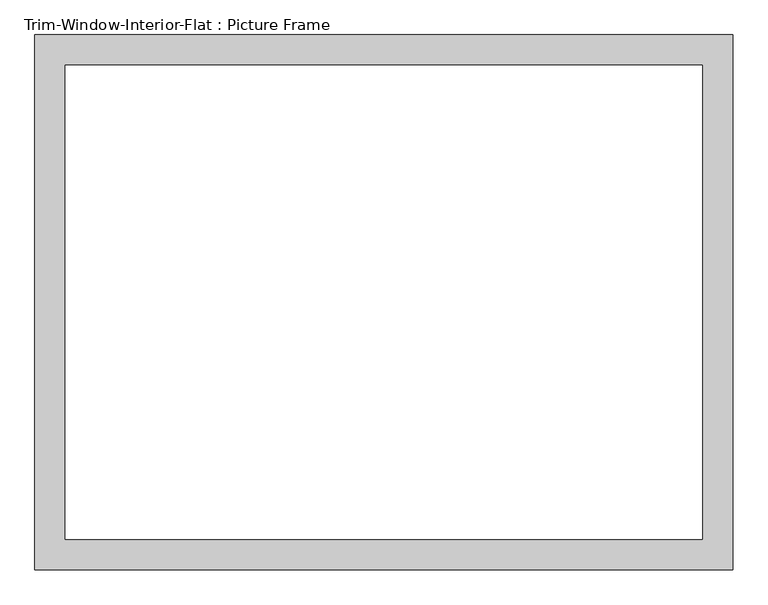
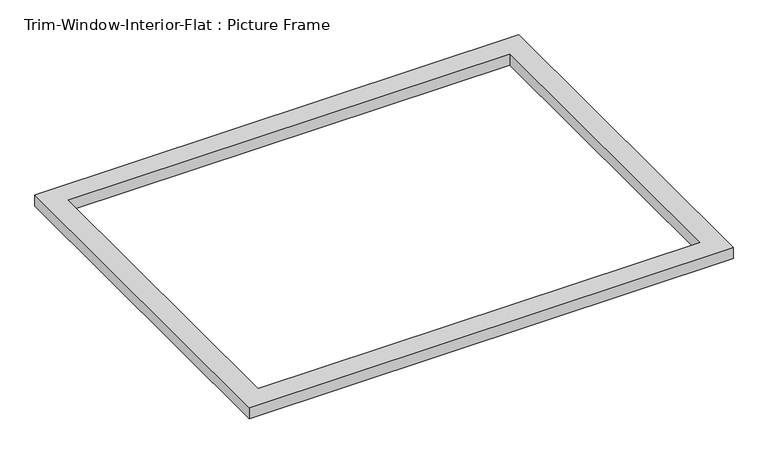
"""IFC4 building model written with IfcOpenShell, lengths in millimetres: proxy geometry, Trim-Window-Interior-Flat : Picture Frame."""

from ifc_helpers import new_model, si_unit, origin, origin_with_axes, place, context, project, spatial, polyline, outline, extrude, source, transform, mapped, element, save


def trim_window_interior_flat_picture_frame_cf1733af(model_context):
    return source(origin(), model_context, "Body", "SweptSolid", [
        extrude(outline(polyline([(654.05, 44.45), (654.05, -958.85), (-654.05, -958.85), (-654.05, 44.45), (654.05, 44.45)]), holes=[polyline([(596.9, -12.7), (-596.9, -12.7), (-596.9, -901.7), (596.9, -901.7), (596.9, -12.7)])]), origin_with_axes(), (0.0, 0.0, 1.0), 31.75),
    ])


if __name__ == "__main__":
    model = new_model("IFC4")
    model_context = context("Model", 3, world=origin())
    ifc_project = project(units=[si_unit("LENGTHUNIT", "METRE", prefix="MILLI")], contexts=[model_context])
    site = spatial("IfcSite", under=ifc_project)
    building = spatial("IfcBuilding", under=site)
    placement = place(None, origin())
    trim_window_interior_flat_picture_frame_shape = trim_window_interior_flat_picture_frame_cf1733af(model_context)
    element("IfcBuildingElementProxy", 1, Name="Trim-Window-Interior-Flat : Picture Frame", ObjectType="Trim-Window-Interior-Flat : Picture Frame", at=placement, inside=building, context=model_context, shape_type="MappedRepresentation", body=[
        mapped(trim_window_interior_flat_picture_frame_shape, transform((0.0, 0.0, 0.0), x_axis=(1.0, 0.0, 0.0), y_axis=(0.0, 1.0, 0.0), z_axis=(0.0, 0.0, 1.0))),
    ])
    save(model, "model.ifc")

# Revit data of these elements
# Type "Trim-Window-Interior-Flat : Picture Frame"
#   Trim Thickness_Picture Frame = 0' - 1 1/4"
#   Trim Width = 0' - 2 1/4"
#   Trim Thickness_with Sill = 0' - 0 3/4"
#   Sill Thickness = 0' - 1 1/4"
#   Opening Width [instance default] = 2' - 0"
#   Opening Height [instance default] = 3' - 0"
#   Default Elevation = 4' - 0"
#   Sill = no
#   Picture Frame = yes
#   Trim Material [instance default] = none
# Element 1 (IfcBuildingElementProxy, "Trim-Window-Interior-Flat : Picture Frame")
#   Opening Width = 4' - 0"
#   Trim Material = Wood - Stained
#   Materials on its faces: "Wood - Stained"
# Materials
#   "Wood - Stained": class "Wood", colour RGB 224 178 126, transparency 0, Cost = 0
